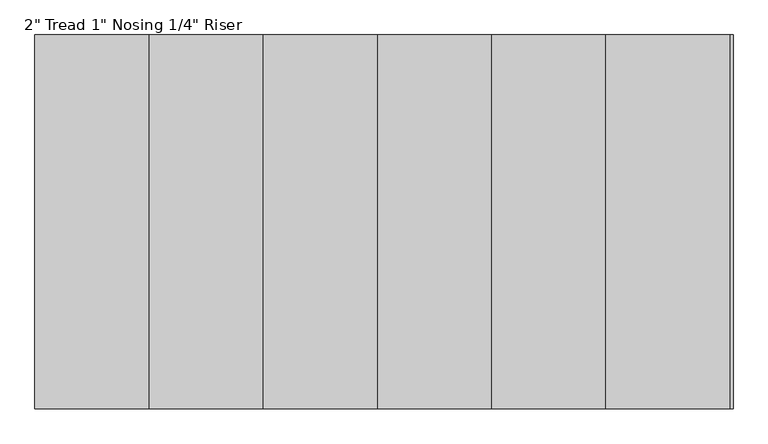
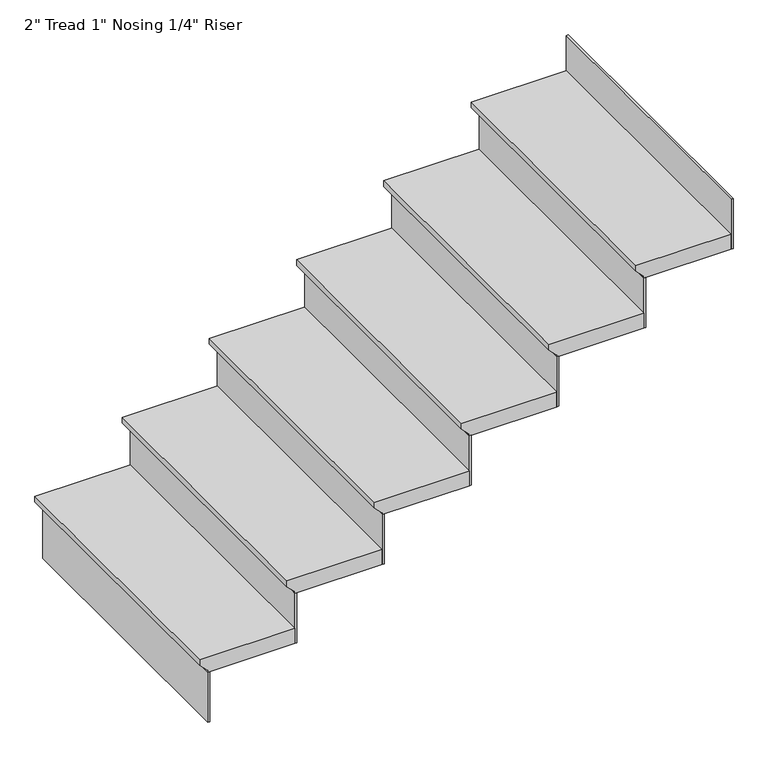
"""IFC4 building model written with IfcOpenShell, lengths in millimetres: stair flight geometry."""

from ifc_helpers import new_model, si_unit, frame, origin, place, context, project, spatial, polyline, outline, extrude, source, transform, mapped, element, save


def stair_flight_8dca3de9(model_context):
    return source(origin(), model_context, "Body", "SweptSolid", [
        extrude(outline(polyline([(5689.6, -8480.0517085), (5689.6, -8784.8517085), (5670.55, -8784.8517085), (5645.15, -8759.4517085), (5638.8, -8759.4517085), (5638.8, -8480.0517085), (5689.6, -8480.0517085)])), frame((0.0, 792.0165128, 0.0), z_axis=(0.0, 1.0, 0.0), x_axis=(0.0, 0.0, 1.0)), (0.0, 0.0, 1.0), 914.4),
        extrude(outline(polyline([(-8753.1017085, 792.0165128), (-8759.4517085, 792.0165128), (-8759.4517085, 1706.4165128), (-8753.1017085, 1706.4165128), (-8753.1017085, 792.0165128)])), frame((0.0, 0.0, 5469.4666667), z_axis=(0.0, 0.0, 1.0), x_axis=(1.0, 0.0, 0.0)), (0.0, 0.0, 1.0), 169.3333333),
        extrude(outline(polyline([(-8473.7017085, 792.0165128), (-8480.0517085, 792.0165128), (-8480.0517085, 1706.4165128), (-8473.7017085, 1706.4165128), (-8473.7017085, 792.0165128)])), frame((0.0, 0.0, 5638.8), z_axis=(0.0, 0.0, 1.0), x_axis=(1.0, 0.0, 0.0)), (0.0, 0.0, 1.0), 169.3333333),
        extrude(outline(polyline([(5858.9333333, -8200.6517085), (5858.9333333, -8505.4517085), (5839.8833333, -8505.4517085), (5814.4833333, -8480.0517085), (5808.1333333, -8480.0517085), (5808.1333333, -8200.6517085), (5858.9333333, -8200.6517085)])), frame((0.0, 792.0165128, 0.0), z_axis=(0.0, 1.0, 0.0), x_axis=(0.0, 0.0, 1.0)), (0.0, 0.0, 1.0), 914.4),
        extrude(outline(polyline([(-8194.3017085, 792.0165128), (-8200.6517085, 792.0165128), (-8200.6517085, 1706.4165128), (-8194.3017085, 1706.4165128), (-8194.3017085, 792.0165128)])), frame((0.0, 0.0, 5808.1333333), z_axis=(0.0, 0.0, 1.0), x_axis=(1.0, 0.0, 0.0)), (0.0, 0.0, 1.0), 169.3333333),
        extrude(outline(polyline([(6028.2666667, -7921.2517085), (6028.2666667, -8226.0517085), (6009.2166667, -8226.0517085), (5983.8166667, -8200.6517085), (5977.4666667, -8200.6517085), (5977.4666667, -7921.2517085), (6028.2666667, -7921.2517085)])), frame((0.0, 792.0165128, 0.0), z_axis=(0.0, 1.0, 0.0), x_axis=(0.0, 0.0, 1.0)), (0.0, 0.0, 1.0), 914.4),
        extrude(outline(polyline([(-7914.9017085, 792.0165128), (-7921.2517085, 792.0165128), (-7921.2517085, 1706.4165128), (-7914.9017085, 1706.4165128), (-7914.9017085, 792.0165128)])), frame((0.0, 0.0, 5977.4666667), z_axis=(0.0, 0.0, 1.0), x_axis=(1.0, 0.0, 0.0)), (0.0, 0.0, 1.0), 169.3333333),
        extrude(outline(polyline([(6197.6, -7641.8517085), (6197.6, -7946.6517085), (6178.55, -7946.6517085), (6153.15, -7921.2517085), (6146.8, -7921.2517085), (6146.8, -7641.8517085), (6197.6, -7641.8517085)])), frame((0.0, 792.0165128, 0.0), z_axis=(0.0, 1.0, 0.0), x_axis=(0.0, 0.0, 1.0)), (0.0, 0.0, 1.0), 914.4),
        extrude(outline(polyline([(-7635.5017085, 792.0165128), (-7641.8517085, 792.0165128), (-7641.8517085, 1706.4165128), (-7635.5017085, 1706.4165128), (-7635.5017085, 792.0165128)])), frame((0.0, 0.0, 6146.8), z_axis=(0.0, 0.0, 1.0), x_axis=(1.0, 0.0, 0.0)), (0.0, 0.0, 1.0), 169.3333333),
        extrude(outline(polyline([(6366.9333333, -7362.4517085), (6366.9333333, -7667.2517085), (6347.8833333, -7667.2517085), (6322.4833333, -7641.8517085), (6316.1333333, -7641.8517085), (6316.1333333, -7362.4517085), (6366.9333333, -7362.4517085)])), frame((0.0, 792.0165128, 0.0), z_axis=(0.0, 1.0, 0.0), x_axis=(0.0, 0.0, 1.0)), (0.0, 0.0, 1.0), 914.4),
        extrude(outline(polyline([(-7356.1017085, 792.0165128), (-7362.4517085, 792.0165128), (-7362.4517085, 1706.4165128), (-7356.1017085, 1706.4165128), (-7356.1017085, 792.0165128)])), frame((0.0, 0.0, 6316.1333333), z_axis=(0.0, 0.0, 1.0), x_axis=(1.0, 0.0, 0.0)), (0.0, 0.0, 1.0), 169.3333333),
        extrude(outline(polyline([(-7076.7017085, 792.0165128), (-7083.0517085, 792.0165128), (-7083.0517085, 1706.4165128), (-7076.7017085, 1706.4165128), (-7076.7017085, 792.0165128)])), frame((0.0, 0.0, 6485.4666667), z_axis=(0.0, 0.0, 1.0), x_axis=(1.0, 0.0, 0.0)), (0.0, 0.0, 1.0), 169.3333333),
        extrude(outline(polyline([(6536.2666667, -7083.0517085), (6536.2666667, -7387.8517085), (6517.2166667, -7387.8517085), (6491.8166667, -7362.4517085), (6485.4666667, -7362.4517085), (6485.4666667, -7083.0517085), (6536.2666667, -7083.0517085)])), frame((0.0, 792.0165128, 0.0), z_axis=(0.0, 1.0, 0.0), x_axis=(0.0, 0.0, 1.0)), (0.0, 0.0, 1.0), 914.4),
    ])


if __name__ == "__main__":
    model = new_model("IFC4")
    model_context = context("Model", 3, world=origin())
    ifc_project = project(units=[si_unit("LENGTHUNIT", "METRE", prefix="MILLI")], contexts=[model_context])
    site = spatial("IfcSite", under=ifc_project)
    building = spatial("IfcBuilding", under=site)
    placement = place(None, origin())
    stair_flight_shape = stair_flight_8dca3de9(model_context)
    element("IfcStairFlight", 1, ObjectType="2\" Tread 1\" Nosing 1/4\" Riser", at=placement, inside=building, context=model_context, shape_type="MappedRepresentation", body=[
        mapped(stair_flight_shape, transform((0.0, 0.0, 0.0), x_axis=(1.0, 0.0, 0.0), y_axis=(0.0, 1.0, 0.0), z_axis=(0.0, 0.0, 1.0))),
    ])
    save(model, "model.ifc")
